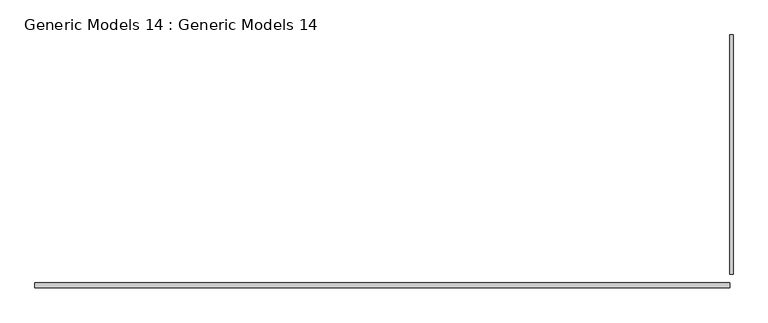
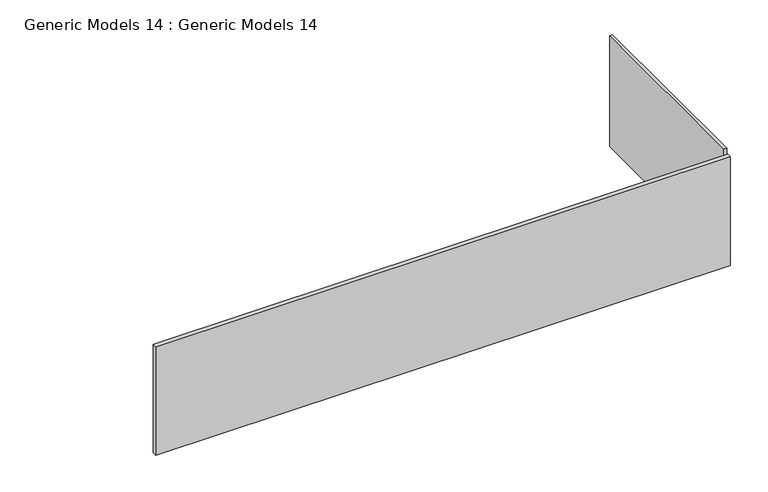
"""IFC4 building model written with IfcOpenShell, lengths in millimetres: proxy geometry, Generic Models 14 : Generic Models 14."""

from ifc_helpers import new_model, si_unit, frame, origin, place, context, project, spatial, polyline, outline, extrude, source, transform, mapped, element, save


def generic_models_14_generic_models_14_d7e62491(model_context):
    return source(origin(), model_context, "Body", "SweptSolid", [
        extrude(outline(polyline([(-12271.2651815, -3418.2388318), (-12283.0500367, -3418.2388318), (-12283.0500367, -2530.6865647), (-12271.2651815, -2530.6865647), (-12271.2651815, -3418.2388318)])), frame((0.0, 0.0, 3980.8624644), z_axis=(0.0, 0.0, 1.0), x_axis=(1.0, 0.0, 0.0)), (0.0, 0.0, 1.0), 527.1995121),
        extrude(outline(polyline([(-12284.1135603, -3449.9627751), (-12284.1135603, -3469.3447554), (-14861.0638674, -3469.3447554), (-14861.0638674, -3449.9627751), (-12284.1135603, -3449.9627751)])), frame((0.0, 0.0, 3987.7146754), z_axis=(0.0, 0.0, 1.0), x_axis=(1.0, 0.0, 0.0)), (0.0, 0.0, 1.0), 516.1760176),
    ])


if __name__ == "__main__":
    model = new_model("IFC4")
    model_context = context("Model", 3, world=origin())
    ifc_project = project(units=[si_unit("LENGTHUNIT", "METRE", prefix="MILLI")], contexts=[model_context])
    site = spatial("IfcSite", under=ifc_project)
    building = spatial("IfcBuilding", under=site)
    placement = place(None, origin())
    generic_models_14_generic_models_14_shape = generic_models_14_generic_models_14_d7e62491(model_context)
    element("IfcBuildingElementProxy", 1, Name="Generic Models 14 : Generic Models 14", ObjectType="Generic Models 14 : Generic Models 14", at=placement, inside=building, context=model_context, shape_type="MappedRepresentation", body=[
        mapped(generic_models_14_generic_models_14_shape, transform((0.0, 0.0, 0.0), x_axis=(1.0, 0.0, 0.0), y_axis=(0.0, 1.0, 0.0), z_axis=(0.0, 0.0, 1.0))),
    ])
    save(model, "model.ifc")

# Revit data of these elements
# Element 1 (IfcBuildingElementProxy, "Generic Models 14 : Generic Models 14")
#   Materials on its faces: "Default Mass Interior Wall", "Default Form"
# Materials
#   "Default Mass Interior Wall": class "Generic", colour RGB 195 229 126, transparency 0, Cost = 0
#   "Default Form": class "Generic", colour RGB 185 189 196, transparency 0.5, Cost = 0
